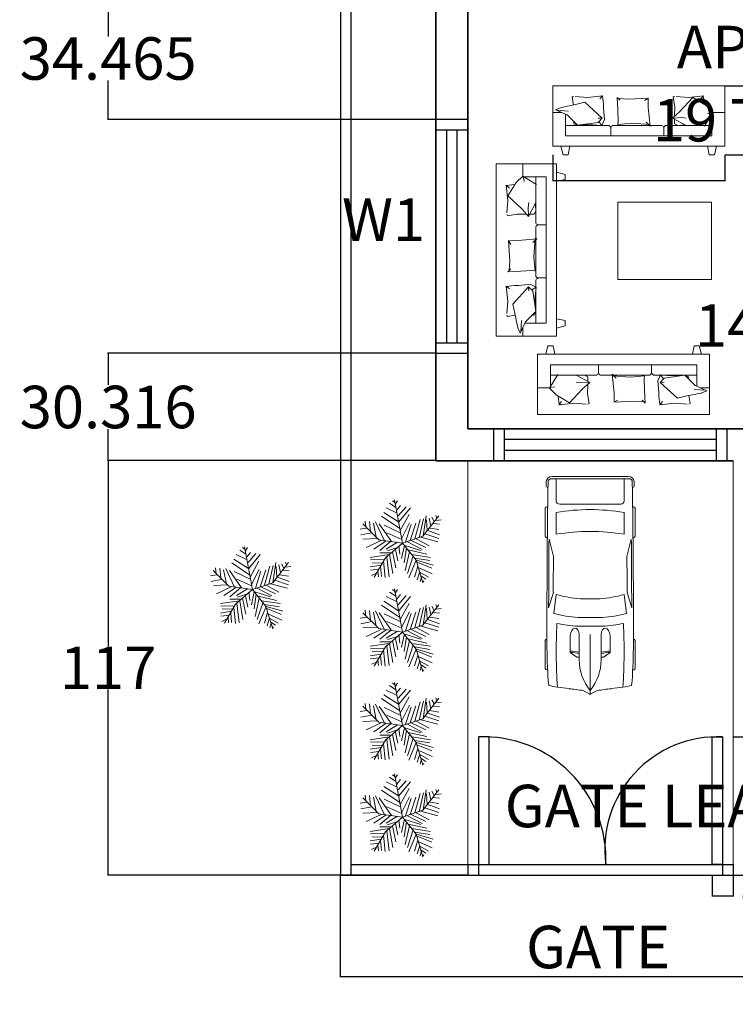
# Model space of a CAD drawing. Units: inches. Extents: x 774 to 1314, y 374 to 930.
# Tile 1 of 5: x 774 to 976, y 374 to 652. Entities that reach past the tile are written whole.
import ezdxf
from ezdxf.enums import TextEntityAlignment as Align

# ---------------------------------------------------------------- set-up
doc = ezdxf.new("R2010")
doc.units = ezdxf.units.IN
doc.header["$MEASUREMENT"] = 0
for name, color, linetype, lineweight in [('A-ANNO-DIMS', 2, 'Continuous', 18), ('A-ANNO-TEXT', 2, 'Continuous', 18), ('A-AREA-IDEN', 2, 'Continuous', 18), ('A-FURN', 8, 'Continuous', 18), ('A-GLAZ', 4, 'Continuous', 18), ('A-WALL', 1, 'Continuous', 35), ('C-PROP', 3, 'Continuous', 25), ('C-VEHC', 8, 'Continuous', 13), ('L-GATE', 6, 'Continuous', 25), ('L-PAVE', 32, 'Continuous', 18), ('L-PLNT', 3, 'Continuous', 13)]:
    doc.layers.add(name, color=color, linetype=linetype, lineweight=lineweight)
doc.layers.add('Layer4', color=4, linetype='Continuous')
doc.styles.get("Standard").update_dxf_attribs({"font": 'arial.ttf'})
doc.dimstyles.get("Standard").update_dxf_attribs({"dimtxt": 12, "dimasz": 0.18, "dimexe": 0.18, "dimexo": 0.0625, "dimgap": 0.09, "dimtad": 0, "dimtih": 1, "dimtoh": 1, "dimdec": 0, "dimzin": 0, "dimdsep": 46, "dimlunit": 4, "dimtxsty": 'Standard', "dimcen": 0.09, "dimadec": 0, "dimazin": 0, "dimtfac": 1, "dimtdec": 0, "dimtofl": 0, "dimtmove": 0, "dimatfit": 3, "dimfxl": 1, "dimtolj": 1, "dimtzin": 0, "dimarcsym": 0})

# ---------------------------------------------------------------- blocks, each defined once
blk = doc.blocks.new('tr')
at = {"layer": 'Layer4'}
for p, q in [((9, 66), (0, 66)), ((9, 63), (0, 63)), ((0, 63), (0, 3)), ((3, 63), (3, 3)), ((6, 3), (6, 63)), ((9, 3), (9, 63)), ((0, 3), (9, 3)), ((0, 0), (9, 0))]:
    blk.add_line(p, q, dxfattribs=at)
blk = doc.blocks.new('A$C684A1F33')
for p, q in [((0, 708), (1769, 708)), ((0, 708), (0, 88)), ((1769, 708), (1769, 88)), ((233, 516), (87, 486)), ((201, 592), (214, 600)), ((215, 513), (201, 592)), ((232, 599), (359, 589)), ((330, 538), (233, 516)), ((508, 377), (330, 538)), ((359, 589), (513, 606)), ((513, 606), (485, 573)), ((490, 603), (511, 604)), ((511, 604), (521, 520)), ((521, 520), (521, 475)), ((669, 458), (662, 589)), ((662, 589), (693, 560)), ((681, 577), (771, 570)), ((771, 570), (984, 581)), ((984, 581), (942, 558)), ((980, 570), (982, 484)), ((1238, 592), (1251, 600)), ((1255, 494), (1238, 592)), ((1269, 599), (1395, 589)), ((1306, 443), (1441, 588)), ((1395, 589), (1550, 606)), ((1441, 588), (1579, 505)), ((1550, 606), (1522, 573)), ((1527, 603), (1548, 604)), ((1548, 604), (1558, 520)), ((1558, 520), (1558, 518)), ((0, 434), (93, 434)), ((87, 486), (30, 462)), ((30, 462), (148, 408)), ((42, 457), (160, 448)), ((133, 415), (133, 195)), ((148, 408), (255, 302)), ((521, 475), (533, 361)), ((674, 340), (669, 458)), ((982, 484), (1001, 292)), ((1230, 377), (1306, 443)), ((1253, 397), (1255, 494)), ((1645, 436), (1559, 294)), ((1579, 505), (1645, 436)), ((1635, 429), (1590, 422)), ((1637, 434), (1637, 195)), ((1637, 434), (1769, 434)), ((216, 318), (216, 340)), ((249, 301), (216, 318)), ((313, 306), (249, 301)), ((255, 302), (467, 332)), ((409, 308), (313, 306)), ((504, 299), (409, 308)), ((498, 377), (467, 375)), ((467, 332), (508, 377)), ((504, 299), (475, 341)), ((533, 361), (504, 299)), ((669, 309), (814, 323)), ((671, 306), (674, 340)), ((814, 323), (1003, 309)), ((1001, 292), (961, 333)), ((1372, 301), (1230, 377)), ((1237, 377), (1323, 381)), ((1252, 318), (1253, 365)), ((1286, 301), (1252, 318)), ((1350, 306), (1286, 301)), ((1323, 381), (1372, 374)), ((1363, 306), (1350, 306)), ((133, 301), (576, 301)), ((598, 277), (598, 195)), ((613, 301), (1122, 301)), ((1144, 277), (1144, 195)), ((1160, 301), (1637, 301)), ((133, 195), (1637, 195)), ((0, 88), (1769, 88)), ((84, 88), (107, 0)), ((177, 88), (160, 0)), ((1592, 88), (1610, 0)), ((1685, 88), (1662, 0)), ((107, 0), (160, 0)), ((1610, 0), (1662, 0))]:
    blk.add_line(p, q)
for points, knots in [([(576, 301), (580, 299), (590, 293), (595, 283), (598, 277)], [15.247039, 15.247039, 15.247039, 15.247039, 32.166322, 53.547435, 53.547435, 53.547435, 53.547435]), ([(598, 276), (599, 282), (602, 291), (610, 298), (613, 301)], [5.353258, 5.353258, 5.353258, 5.353258, 23.098733, 39.167876, 39.167876, 39.167876, 39.167876]), ([(1122, 301), (1127, 299), (1136, 293), (1141, 283), (1144, 277)], [15.247039, 15.247039, 15.247039, 15.247039, 32.166322, 53.547435, 53.547435, 53.547435, 53.547435]), ([(1144, 276), (1145, 282), (1149, 291), (1156, 298), (1160, 301)], [5.353258, 5.353258, 5.353258, 5.353258, 23.098733, 39.167876, 39.167876, 39.167876, 39.167876])]:
    blk.add_open_spline(points, degree=3, knots=knots)
blk = doc.blocks.new('*U12')
for p, q in [((21.1, 37.41), (21.1, 36.83)), ((46.55, 38.89), (22.35, 38.89)), ((47.8, 37.39), (47.8, 37.41)), ((87.99, 31.87), (74.76, 35.92)), ((134.31, 35.6), (119.29, 31.78)), ((135.45, 37.07), (135.45, 37.41)), ((136.7, 38.89), (160.9, 38.89)), ((162.15, 37.41), (162.15, 36.77)), ((70.03, 31.54), (86.41, 29.35)), ((138.42, 29.35), (157.25, 29.35)), ((164.52, 26.39), (164.52, -26.39)), ((186.47, 29.35), (167.01, 29.35)), ((186.47, -33.5), (186.47, 33.5)), ((188.4, -32.76), (188.4, 32.76)), ((32.27, 11.63), (36.13, 17.17)), ((36.13, 17.17), (50.94, 17.17)), ((29.77, 9.51), (51.68, 9.51)), ((32.12, 9.51), (32.12, 11.15)), ((58.92, -10.77), (58.92, 10.77)), ((66.55, -10.53), (66.55, 10.53)), ((186.47, -10.53), (186.47, 10.53)), ((3.27, 6.13), (0.1, 0.41)), ((82.74, 8.5), (82.74, -8.5)), ((0, 0), (51.68, 0)), ((0.1, -0.41), (3.27, -6.13)), ((29.77, -9.51), (51.68, -9.51)), ((32.12, -9.51), (32.12, -11.15)), ((32.27, -11.63), (36.13, -17.17)), ((36.13, -17.17), (50.94, -17.17)), ((86.41, -29.35), (70.03, -31.54)), ((87.99, -31.87), (74.76, -35.92)), ((134.31, -35.6), (119.29, -31.78)), ((157.25, -29.35), (138.42, -29.35)), ((167.01, -29.35), (186.47, -29.35)), ((21.1, -37.41), (21.1, -36.83)), ((46.55, -38.89), (22.35, -38.89)), ((47.8, -37.39), (47.8, -37.41)), ((135.45, -37.07), (135.45, -37.41)), ((136.7, -38.89), (160.9, -38.89)), ((162.15, -37.41), (162.15, -36.77))]:
    blk.add_line(p, q)
for centre, major_axis, ratio, start_param, end_param in [((266.03, -27.52), (0, 313.31), 0.842304, 1.367076, 1.39176), ((41.19, -490.86), (0, 528.23), 0.842304, 0.00281, 0.075598), ((22.35, 37.41), (0, -1.48), 0.842304, 3.141593, 4.712389), ((64.48, -10555.62), (0, 10593.03), 0.842304, -0.013397, 0.002797), ((46.55, 37.41), (0, 1.48), 0.842304, -1.570796, 0), ((64.48, -10555.62), (0, -10591.55), 0.842304, 3.133765, 3.140441), ((136.7, 37.41), (0, -1.48), 0.842304, 3.141593, 4.712389), ((160.9, 37.41), (0, 1.48), 0.842304, -1.570796, 0), ((180.63, 35.84), (0, 2.22), 0.842304, -0.013017, 1.249894), ((64.48, -10556.36), (0, 10595.31), 0.842304, -0.013397, -0.013017), ((183.98, 33.5), (0, -2.96), 0.842304, 1.570796, 3.128196), ((183.98, 32.76), (0, -5.25), 0.842304, 1.570796, 3.128196), ((259.18, -27.52), (0, -305.3), 0.842304, 4.528606, 4.561838), ((37.47, -593.96), (0, -623.33), 0.842304, 3.096046, 3.200911), ((134.4, 5.39), (0, -89.78), 0.842304, 4.449482, 4.652344), ((135.29, 5.39), (0, 81.77), 0.842304, 1.245306, 1.50788), ((149.6, 2.8), (0, -79.58), 0.842304, 4.372215, 4.640744), ((95.79, -3666.35), (0, -3698.24), 0.842304, 3.134049, 3.144098), ((17.08, 0), (0, 147.02), 0.842304, 4.511394, 4.913384), ((35.91, 0), (0, 147.02), 0.842304, 4.511394, 4.913384), ((167.01, 26.39), (0, 2.96), 0.842304, 0, 1.570796), ((-204.49, 52.4), (0, -250.96), 0.842304, 1.385369, 1.434372), ((13.04, 17.01), (0, 27.42), 0.842304, 4.435146, 4.718221), ((14.2, 17.01), (0, 27.42), 0.842304, 4.435146, 4.718221), ((50.79, 13.34), (6.34, -0.36), 0.603834, -1.395552, 1.581315), ((29.77, -46.66), (0, 56.17), 0.842304, 0, 0.590319), ((32.75, 11.15), (0, 0.74), 0.842304, 0.879714, 1.570796), ((0.62, 0), (0, -0.74), 0.842304, 4.131459, 5.293319), ((-204.49, -52.4), (0, 250.96), 0.842304, -1.434372, -1.385369), ((29.77, 46.66), (0, 56.17), 0.842304, 2.551274, 3.141593), ((149.6, -2.8), (0, -79.58), 0.842304, -1.499151, -1.230623), ((32.75, -11.15), (0, -0.74), 0.842304, 4.712389, 5.403472), ((13.04, -17.01), (0, -27.42), 0.842304, 1.564964, 1.848039), ((14.2, -17.01), (0, -27.42), 0.842304, 1.564964, 1.848039), ((134.4, -5.39), (0, -89.78), 0.842304, -1.510751, -1.307889), ((135.29, -5.39), (0, -81.77), 0.842304, -1.50788, -1.245306), ((259.18, 27.52), (0, 305.3), 0.842304, 1.721348, 1.754579), ((266.03, 27.52), (0, 313.31), 0.842304, 1.749832, 1.774517), ((37.47, 593.96), (0, -623.33), 0.842304, -0.059319, 0.045547), ((95.79, 3666.35), (0, -3698.24), 0.842304, -0.002505, 0.007544), ((167.01, -26.39), (0, -2.96), 0.842304, 4.712389, 6.283185), ((183.98, -33.5), (0, 2.96), 0.842304, 3.15499, 4.712389), ((183.98, -32.76), (0, -5.25), 0.842304, 0.013397, 1.570796), ((41.19, 490.86), (0, -528.23), 0.842304, -0.075598, -0.00281), ((22.35, -37.41), (0, 1.48), 0.842304, 1.570796, 3.141593), ((64.48, 10555.62), (0, 10593.03), 0.842304, 3.138796, 3.15499), ((46.55, -37.41), (0, -1.48), 0.842304, 0, 1.570796), ((64.48, 10555.62), (0, -10591.55), 0.842304, 0.001152, 0.007828), ((136.7, -37.41), (0, -1.48), 0.842304, -1.570796, 0), ((160.9, -37.41), (0, 1.48), 0.842304, 3.141593, 4.712389), ((180.63, -35.84), (0, -2.22), 0.842304, -1.249894, 0.013017), ((64.48, 10556.36), (0, 10595.31), 0.842304, 3.15461, 3.15499)]:
    blk.add_ellipse(centre, major_axis=major_axis, ratio=ratio, start_param=start_param, end_param=end_param)
at = {"extrusion": (0, 0, -1)}
blk.add_ellipse((50.79, -13.34), major_axis=(6.34, 0.36), ratio=0.603834, start_param=-1.395552, end_param=1.581315, dxfattribs=at)
blk = doc.blocks.new('*U14')
for p, q in [((-8.737, 47.138), (-17.069, 52.711)), ((-10.186, 53.64), (-13.084, 55.962)), ((0, 0), (-10.5, 57)), ((-9.099, 51.782), (-6.563, 55.962)), ((-5.114, 28.097), (-24.676, 40.636)), ((-7.288, 39.707), (-21.778, 46.673)), ((-7.65, 43.423), (-2.578, 49.46)), ((-5.839, 35.992), (4.667, 48.067)), ((-5.114, 27.632), (10.463, 46.673)), ((-48.585, 21.131), (-49.309, 29.026)), ((-43.513, 28.561), (-42.427, 15.558)), ((-38.442, 26.239), (-34.819, 7.663)), ((-35.544, 28.097), (-24.314, 3.947)), ((-3.665, 19.273), (-27.574, 35.527)), ((-2.941, 16.486), (8.652, 37.85)), ((-1.129, 6.734), (9.014, 26.704)), ((10.101, 3.483), (17.708, 26.239)), ((16.259, 5.805), (23.142, 31.348)), ((22.055, 7.198), (27.489, 32.277)), ((27, 9), (48, 36)), ((27.127, 9.056), (31.112, 35.992)), ((31.836, 30.883), (32.561, 16.486)), ((35.096, 32.741), (37.27, 22.524)), ((38.719, 34.134), (41.979, 28.561)), ((43.791, 29.954), (51.036, 30.883)), ((44.153, 36.456), (45.239, 32.741)), ((-47.498, 19.737), (-55.83, 18.344)), ((-40.615, 13.7), (-55.105, 10.913)), ((-31.5, 4.5), (-52.5, 25.5)), ((-14.533, 2.09), (-30.834, 25.31)), ((-24.314, 23.917), (-2.941, 13.7)), ((-20.691, 13.7), (-1.129, 4.876)), ((3.942, 1.625), (11.187, 24.381)), ((33.285, 16.486), (48.862, 10.913)), ((36.183, 19.737), (48.137, 17.88)), ((40.53, 25.775), (48.862, 24.846)), ((-33.37, 6.269), (-52.207, 5.34)), ((-28.299, 3.483), (-47.86, -5.805)), ((-21.416, 3.018), (-38.079, -8.128)), ((0, 0), (-31.5, 4.5)), ((-15.982, 2.09), (-30.11, -9.521)), ((0, 0), (-22.5, -19.5)), ((-6.563, 1.161), (-21.416, -8.128)), ((0, 0), (27, 9)), ((0, 0), (18, -22.5)), ((6.478, 1.625), (26.04, -8.592)), ((11.187, 3.483), (30.749, -5.805)), ((18.07, 5.805), (35.096, -3.483)), ((24.229, 7.663), (46.688, 1.625)), ((29.662, 12.307), (48.137, 6.269)), ((-15.257, -12.772), (-30.11, -12.772)), ((-6.563, -5.805), (-19.967, -9.985)), ((-13.446, -11.378), (-8.737, -32.741)), ((-9.461, -8.592), (-6.201, -23.453)), ((-4.752, -3.483), (-3.665, -14.629)), ((2.493, -3.019), (-1.491, -20.202)), ((1.769, -2.555), (24.229, -9.521)), ((5.029, -6.27), (2.131, -25.775)), ((9.014, -11.378), (3.58, -35.992)), ((7.565, -9.056), (32.198, -14.629)), ((-17.431, -15.094), (-42.789, -18.809)), ((-24.314, -21.596), (-42.427, -22.06)), ((-26.849, -26.24), (-40.253, -25.775)), ((-22.5, -19.5), (-37.5, -45)), ((-25.038, -23.918), (-22.865, -45.281)), ((-20.691, -18.345), (-17.793, -44.352)), ((-17.069, -15.094), (-12.721, -40.172)), ((14.085, -16.951), (6.478, -40.172)), ((18.07, -22.524), (8.289, -45.745)), ((12.274, -15.094), (36.907, -18.809)), ((16.259, -19.738), (36.183, -22.989)), ((18, -22.5), (27, -52.5)), ((18.433, -22.524), (40.53, -29.026)), ((19.157, -25.311), (38.719, -33.206)), ((-28.299, -29.026), (-42.789, -31.348)), ((-30.834, -34.135), (-42.427, -35.528)), ((-32.646, -36.921), (-31.921, -44.352)), ((-29.023, -30.884), (-27.936, -43.887)), ((20.244, -30.419), (15.897, -44.816)), ((22.78, -37.85), (19.519, -48.532)), ((21.331, -32.741), (39.081, -40.636)), ((22.78, -38.314), (34.372, -44.816)), ((-34.457, -39.708), (-40.978, -42.494)), ((24.591, -45.745), (23.142, -50.854)), ((24.591, -43.423), (30.749, -47.603)), ((26.764, -49.925), (28.213, -50.854))]:
    blk.add_line(p, q)
blk = doc.blocks.new('*U16')
for p, q in [((-221.9198, 1197.3052), (-433.5526, 1338.8594)), ((-258.7244, 1362.456), (-332.3336, 1421.4348)), ((0, 0), (-266.7, 1447.8)), ((-231.1146, 1315.2628), (-166.7002, 1421.4348)), ((-129.8956, 713.6638), (-626.7704, 1032.1544)), ((-185.1152, 1008.5578), (-553.1612, 1185.4942)), ((-194.31, 1102.9442), (-65.4812, 1256.284)), ((-148.3106, 914.1968), (118.5418, 1220.9018)), ((-129.8956, 701.8528), (265.7602, 1185.4942)), ((-1234.059, 536.7274), (-1252.4486, 737.2604)), ((-1105.2302, 725.4494), (-1077.6458, 395.1732)), ((-902.8176, 713.6638), (-617.5756, 100.2538)), ((-93.091, 489.5342), (-700.3796, 902.3858)), ((-74.7014, 418.7444), (219.7608, 961.39)), ((-28.6766, 171.0436), (228.9556, 678.2816)), ((412.9786, 147.447), (587.8068, 796.2392)), ((560.197, 182.8292), (698.2206, 819.8358)), ((685.8, 228.6), (1219.2, 914.4)), ((689.0258, 230.0224), (790.2448, 914.1968)), ((808.6344, 784.4282), (827.0494, 418.7444)), ((891.4384, 831.6214), (946.658, 572.1096)), ((983.4626, 867.0036), (1066.2666, 725.4494)), ((1112.2914, 760.8316), (1296.3144, 784.4282)), ((1121.4862, 925.9824), (1149.0706, 831.6214)), ((-1206.4492, 501.3198), (-1418.082, 465.9376)), ((-1031.621, 347.98), (-1399.667, 277.1902)), ((-800.1, 114.3), (-1333.5, 647.7)), ((-976.4268, 666.4706), (-884.4026, 194.6402)), ((-369.1382, 53.086), (-783.1836, 642.874)), ((-617.5756, 607.4918), (-74.7014, 347.98)), ((-525.5514, 347.98), (-28.6766, 123.8504)), ((100.1268, 41.275), (284.1498, 619.2774)), ((256.5654, 88.4682), (449.7832, 666.4706)), ((845.439, 418.7444), (1241.0948, 277.1902)), ((919.0482, 501.3198), (1222.6798, 454.152)), ((1029.462, 654.685), (1241.0948, 631.0884)), ((-847.598, 159.2326), (-1326.0578, 135.636)), ((-718.7946, 88.4682), (-1215.644, -147.447)), ((-543.9664, 76.6572), (-967.2066, -206.4512)), ((0, 0), (-800.1, 114.3)), ((-405.9428, 53.086), (-764.794, -241.8334)), ((0, 0), (-571.5, -495.3)), ((-166.7002, 29.4894), (-543.9664, -206.4512)), ((0, 0), (685.8, 228.6)), ((0, 0), (457.2, -571.5)), ((164.5412, 41.275), (661.416, -218.2368)), ((284.1498, 88.4682), (781.0246, -147.447)), ((458.978, 147.447), (891.4384, -88.4682)), ((615.4166, 194.6402), (1185.8752, 41.275)), ((753.4148, 312.5978), (1222.6798, 159.2326)), ((-387.5278, -324.4088), (-764.794, -324.4088)), ((-166.7002, -147.447), (-507.1618, -253.619)), ((-341.5284, -289.0012), (-221.9198, -831.6214)), ((-240.3094, -218.2368), (-157.5054, -595.7062)), ((-120.7008, -88.4682), (-93.091, -371.5766)), ((63.3222, -76.6826), (-37.8714, -513.1308)), ((44.9326, -64.897), (615.4166, -241.8334)), ((127.7366, -159.258), (54.1274, -654.685)), ((228.9556, -289.0012), (90.932, -914.1968)), ((192.151, -230.0224), (817.8292, -371.5766)), ((-442.7474, -383.3876), (-1086.8406, -477.7486)), ((-617.5756, -548.5384), (-1077.6458, -560.324)), ((-681.9646, -666.496), (-1022.4262, -654.685)), ((-571.5, -495.3), (-952.5, -1143)), ((-635.9652, -607.5172), (-580.771, -1150.1374)), ((-525.5514, -465.963), (-451.9422, -1126.5408)), ((-433.5526, -383.3876), (-323.1134, -1020.3688)), ((357.759, -430.5554), (164.5412, -1020.3688)), ((458.978, -572.1096), (210.5406, -1161.923)), ((311.7596, -383.3876), (937.4378, -477.7486)), ((412.9786, -501.3452), (919.0482, -583.9206)), ((457.2, -571.5), (685.8, -1333.5)), ((468.1982, -572.1096), (1029.462, -737.2604)), ((486.5878, -642.8994), (983.4626, -843.4324)), ((-718.7946, -737.2604), (-1086.8406, -796.2392)), ((-783.1836, -867.029), (-1077.6458, -902.4112)), ((-829.2084, -937.7934), (-810.7934, -1126.5408)), ((-737.1842, -784.4536), (-709.5744, -1114.7298)), ((514.1976, -772.6426), (403.7838, -1138.3264)), ((578.612, -961.39), (495.7826, -1232.7128)), ((541.8074, -831.6214), (992.6574, -1032.1544)), ((578.612, -973.1756), (873.0488, -1138.3264)), ((-875.2078, -1008.5832), (-1040.8412, -1079.3476)), ((624.6114, -1161.923), (587.8068, -1291.6916)), ((624.6114, -1102.9442), (781.0246, -1209.1162)), ((679.8056, -1268.095), (716.6102, -1291.6916))]:
    blk.add_line(p, q)
blk = doc.blocks.new('GATE-LEAF-36IN')
for p, q in [((3, 3), (3, 0)), ((6, 3), (6, 0))]:
    blk.add_line(p, q)
blk.add_lwpolyline([(3, 3), (0, 3), (0, 39), (3, 39)], close=True)
blk = doc.blocks.new('*D33')
at = {"layer": 'A-ANNO-DIMS', "color": 0, "lineweight": -2, "transparency": 16777216}
for p, q in [((975.4, 449.57), (981.36, 449.57)), ((981.18, 449.39), (981.18, 436.36)), ((981.18, 410.75), (981.18, 423.77)), ((975.4, 410.57), (981.36, 410.57))]:
    blk.add_line(p, q, dxfattribs=at)
at = {"layer": 'A-ANNO-DIMS', "color": 0, "transparency": 16777216}
for points in [[(981.15, 449.39), (981.21, 449.39), (981.18, 449.57)], [(981.15, 410.75), (981.21, 410.75), (981.18, 410.57)]]:
    blk.add_solid(points, dxfattribs=at)
at = {"layer": 'Defpoints', "color": 0, "transparency": 16777216}
for p in [(975.33, 449.57), (981.18, 449.57), (975.33, 410.57)]:
    blk.add_point(p, dxfattribs=at)
at = {"layer": 'A-ANNO-DIMS', "color": 0, "transparency": 16777216, "insert": (981.18, 430.07), "char_height": 12, "attachment_point": 5}
blk.add_mtext('\\A1;GATE LEAF 39 TYP.', dxfattribs=at)
blk = doc.blocks.new('*D34')
at = {"layer": 'A-ANNO-DIMS', "color": 0, "lineweight": -2, "transparency": 16777216}
for p, q in [((969.33, 410.5), (969.33, 404.54)), ((975.33, 410.5), (975.33, 404.54)), ((969.51, 404.72), (975.15, 404.72)), ((975.33, 404.72), (975.51, 404.72))]:
    blk.add_line(p, q, dxfattribs=at)
at = {"layer": 'A-ANNO-DIMS', "color": 0, "transparency": 16777216}
for points in [[(969.51, 404.75), (969.51, 404.69), (969.33, 404.72)], [(975.15, 404.75), (975.15, 404.69), (975.33, 404.72)]]:
    blk.add_solid(points, dxfattribs=at)
at = {"layer": 'Defpoints', "color": 0, "transparency": 16777216}
for p in [(969.33, 410.57), (975.33, 410.57), (975.33, 404.72)]:
    blk.add_point(p, dxfattribs=at)
at = {"layer": 'A-ANNO-DIMS', "color": 0, "transparency": 16777216, "insert": (1000.18, 404.72), "char_height": 12, "attachment_point": 5}
blk.add_mtext('\\A1;6 TYP.', dxfattribs=at)
blk = doc.blocks.new('*D37')
at = {"layer": 'A-ANNO-DIMS', "color": 0, "lineweight": -2, "transparency": 16777216}
for p, q in [((924.33, 613.89), (924.33, 606.48)), ((972.96, 613.89), (972.96, 606.48)), ((924.51, 606.66), (972.78, 606.66)), ((972.96, 606.66), (973.14, 606.66))]:
    blk.add_line(p, q, dxfattribs=at)
at = {"layer": 'A-ANNO-DIMS', "color": 0, "transparency": 16777216}
for points in [[(924.51, 606.69), (924.51, 606.63), (924.33, 606.66)], [(972.78, 606.69), (972.78, 606.63), (972.96, 606.66)]]:
    blk.add_solid(points, dxfattribs=at)
at = {"layer": 'Defpoints', "color": 0, "transparency": 16777216}
for p in [(924.33, 613.95), (972.96, 613.95), (972.96, 606.66)]:
    blk.add_point(p, dxfattribs=at)
at = {"layer": 'A-ANNO-DIMS', "color": 0, "transparency": 16777216, "insert": (1027.55, 606.66), "char_height": 12, "attachment_point": 5}
blk.add_mtext('\\A1;SOFA 49 TYP.', dxfattribs=at)
blk = doc.blocks.new('*D38')
at = {"layer": 'A-ANNO-DIMS', "color": 0, "lineweight": -2, "transparency": 16777216}
for p, q in [((973.02, 633.4), (980.43, 633.4)), ((980.25, 633.22), (980.25, 629.89)), ((980.25, 614.13), (980.25, 617.46)), ((973.02, 613.95), (980.43, 613.95))]:
    blk.add_line(p, q, dxfattribs=at)
at = {"layer": 'A-ANNO-DIMS', "color": 0, "transparency": 16777216}
for points in [[(980.22, 633.22), (980.28, 633.22), (980.25, 633.4)], [(980.22, 614.13), (980.28, 614.13), (980.25, 613.95)]]:
    blk.add_solid(points, dxfattribs=at)
at = {"layer": 'Defpoints', "color": 0, "transparency": 16777216}
for p in [(972.96, 633.4), (980.25, 633.4), (972.96, 613.95)]:
    blk.add_point(p, dxfattribs=at)
at = {"layer": 'A-ANNO-DIMS', "color": 0, "transparency": 16777216, "insert": (980.25, 623.68), "char_height": 12, "attachment_point": 5}
blk.add_mtext('\\A1;19 TYP.', dxfattribs=at)
blk = doc.blocks.new('*D51')
at = {"layer": 'A-ANNO-DIMS', "color": 0, "lineweight": -2, "transparency": 16777216}
for p, q in [((1072.03, 644.35), (1071.85, 644.35)), ((1072.03, 640.32), (1072.03, 644.53)), ((1099.12, 644.35), (1072.21, 644.35)), ((1099.3, 640.32), (1099.3, 644.53))]:
    blk.add_line(p, q, dxfattribs=at)
at = {"layer": 'A-ANNO-DIMS', "color": 0, "transparency": 16777216}
for points in [[(1072.21, 644.38), (1072.21, 644.32), (1072.03, 644.35)], [(1099.12, 644.38), (1099.12, 644.32), (1099.3, 644.35)]]:
    blk.add_solid(points, dxfattribs=at)
at = {"layer": 'Defpoints', "color": 0, "transparency": 16777216}
for p in [(1072.03, 644.35), (1072.03, 640.25), (1099.3, 640.25)]:
    blk.add_point(p, dxfattribs=at)
at = {"layer": 'A-ANNO-DIMS', "color": 0, "transparency": 16777216, "insert": (1013.43, 644.35), "char_height": 12, "attachment_point": 5}
blk.add_mtext('\\A1;APPLIANCE 27', dxfattribs=at)
blk = doc.blocks.new('*D53')
at = {"layer": 'A-ANNO-DIMS', "color": 0, "lineweight": -2, "transparency": 16777216}
for p, q in [((864.33, 410.5), (864.33, 381.78)), ((1230.33, 410.5), (1230.33, 381.78)), ((864.51, 381.96), (1034, 381.96)), ((1230.15, 381.96), (1060.67, 381.96))]:
    blk.add_line(p, q, dxfattribs=at)
at = {"layer": 'A-ANNO-DIMS', "color": 0, "transparency": 16777216}
for points in [[(864.51, 381.99), (864.51, 381.93), (864.33, 381.96)], [(1230.15, 381.99), (1230.15, 381.93), (1230.33, 381.96)]]:
    blk.add_solid(points, dxfattribs=at)
at = {"layer": 'Defpoints', "color": 0, "transparency": 16777216}
for p in [(864.33, 410.57), (1230.33, 410.57), (1230.33, 381.96)]:
    blk.add_point(p, dxfattribs=at)
at = {"layer": 'A-ANNO-DIMS', "color": 0, "transparency": 16777216, "insert": (1047.33, 381.96), "char_height": 12, "attachment_point": 5}
blk.add_mtext('\\A1;366', dxfattribs=at)
blk = doc.blocks.new('*D61')
at = {"layer": 'A-ANNO-DIMS', "color": 0, "lineweight": -2, "transparency": 16777216}
for p, q in [((891.27, 527.57), (798.56, 527.57)), ((798.74, 527.39), (798.74, 475.18)), ((798.74, 410.75), (798.74, 462.95)), ((900.27, 410.57), (798.56, 410.57))]:
    blk.add_line(p, q, dxfattribs=at)
at = {"layer": 'A-ANNO-DIMS', "color": 0, "transparency": 16777216}
for points in [[(798.71, 527.39), (798.77, 527.39), (798.74, 527.57)], [(798.71, 410.75), (798.77, 410.75), (798.74, 410.57)]]:
    blk.add_solid(points, dxfattribs=at)
at = {"layer": 'Defpoints', "color": 0, "transparency": 16777216}
for p in [(798.74, 527.57), (891.33, 527.57), (900.33, 410.57)]:
    blk.add_point(p, dxfattribs=at)
at = {"layer": 'A-ANNO-DIMS', "color": 0, "transparency": 16777216, "insert": (798.74, 469.07), "char_height": 12, "attachment_point": 5}
blk.add_mtext('\\A1;117', dxfattribs=at)
blk = doc.blocks.new('*D62')
at = {"layer": 'A-ANNO-DIMS', "color": 0, "lineweight": -2, "transparency": 16777216}
for p, q in [((891.27, 557.88), (798.56, 557.88)), ((798.74, 557.7), (798.74, 548.94)), ((798.74, 527.75), (798.74, 536.5)), ((891.27, 527.57), (798.56, 527.57))]:
    blk.add_line(p, q, dxfattribs=at)
at = {"layer": 'A-ANNO-DIMS', "color": 0, "transparency": 16777216}
for points in [[(798.71, 557.7), (798.77, 557.7), (798.74, 557.88)], [(798.71, 527.75), (798.77, 527.75), (798.74, 527.57)]]:
    blk.add_solid(points, dxfattribs=at)
at = {"layer": 'Defpoints', "color": 0, "transparency": 16777216}
for p in [(798.74, 557.88), (891.33, 557.88), (891.33, 527.57)]:
    blk.add_point(p, dxfattribs=at)
at = {"layer": 'A-ANNO-DIMS', "color": 0, "transparency": 16777216, "insert": (798.74, 542.72), "char_height": 12, "attachment_point": 5}
blk.add_mtext('\\A1;30.316', dxfattribs=at)
blk = doc.blocks.new('*D63')
at = {"layer": 'A-ANNO-DIMS', "color": 0, "lineweight": -2, "transparency": 16777216}
for p, q in [((891.27, 658.35), (798.56, 658.35)), ((798.74, 658.17), (798.74, 647.34)), ((798.74, 624.06), (798.74, 634.89)), ((891.27, 623.88), (798.56, 623.88))]:
    blk.add_line(p, q, dxfattribs=at)
at = {"layer": 'A-ANNO-DIMS', "color": 0, "transparency": 16777216}
for points in [[(798.71, 658.17), (798.77, 658.17), (798.74, 658.35)], [(798.71, 624.06), (798.77, 624.06), (798.74, 623.88)]]:
    blk.add_solid(points, dxfattribs=at)
at = {"layer": 'Defpoints', "color": 0, "transparency": 16777216}
for p in [(798.74, 658.35), (891.33, 658.35), (891.33, 623.88)]:
    blk.add_point(p, dxfattribs=at)
at = {"layer": 'A-ANNO-DIMS', "color": 0, "transparency": 16777216, "insert": (798.74, 641.11), "char_height": 12, "attachment_point": 5}
blk.add_mtext('\\A1;34.465', dxfattribs=at)

msp = doc.modelspace()

# ---------------------------------------------------------------- linework, layer by layer
at = {"layer": 'A-FURN'}
msp.add_lwpolyline([(942.7268, 578.7015), (969.1941, 578.7015), (969.1941, 600.5862), (942.7268, 600.5862)], close=True, dxfattribs=at)
at = {"layer": 'A-WALL'}
for p, q in [((900.3347, 734.5656), (900.3347, 536.5656)), ((984.3347, 536.5656), (900.3347, 536.5656)), ((975.3347, 527.5656), (891.3347, 527.5656))]:
    msp.add_line(p, q, dxfattribs=at)
msp.add_lwpolyline([(1203.3347, 740.5656), (1203.3347, 869.5656), (891.3347, 869.5656), (891.3347, 527.5656)], dxfattribs=at)
at = {"layer": 'C-PROP'}
msp.add_line((867.3347, 413.5656), (867.3347, 410.5656), dxfattribs=at)
msp.add_lwpolyline([(864.3347, 410.5656), (1230.3347, 410.5656), (1230.3347, 896.5656), (864.3347, 896.5656)], close=True, dxfattribs=at)
for points in [[(1227.3347, 740.5656), (1227.3347, 893.5656), (867.3347, 893.5656), (867.3347, 413.5656), (975.3347, 413.5656)], [(900.3347, 413.5656), (975.3347, 413.5656)]]:
    msp.add_lwpolyline(points, dxfattribs=at)
at = {"layer": 'L-GATE'}
for centre, radius, start, end in [((904.8347, 415.0656), 34.5326, 357.510447, 92.489553), ((970.8347, 417.8156), 31.7854, 87.295124, 187.683982)]:
    msp.add_arc(centre, radius, start, end, dxfattribs=at)
at = {"layer": 'L-PAVE'}
for p, q in [((900.3347, 527.5656), (900.3347, 413.5656)), ((975.3347, 413.5656), (975.3347, 527.5656))]:
    msp.add_line(p, q, dxfattribs=at)

# ---------------------------------------------------------------- block references
at = {"layer": 'A-FURN', "xscale": 0.0274825048750847, "yscale": 0.0274825048750847, "zscale": 0.0274825048750847}
msp.add_blockref('A$C684A1F33', (924.3264, 613.9496), dxfattribs=at)
for p, rotation in [((927.8424, 562.7095), 90), ((968.6583, 560.0203), 180.0000000000001)]:
    msp.add_blockref('A$C684A1F33', p, dxfattribs=dict(at, rotation=rotation))
at = {"layer": 'A-GLAZ'}
msp.add_blockref('tr', (891.3347, 557.8818), dxfattribs=at)
at = {"layer": 'A-GLAZ', "rotation": 270}
msp.add_blockref('tr', (907.6221, 536.5656), dxfattribs=at)
at = {"layer": 'C-VEHC', "xscale": 0.3265334135073655, "yscale": 0.3265334135073655, "zscale": 0.3265334135073655, "rotation": 90}
msp.add_blockref('*U12', (934.9117, 461.5901), dxfattribs=at)
at = {"layer": 'L-GATE', "extrusion": (0, 0, -1), "zscale": -1}
msp.add_blockref('GATE-LEAF-36IN', (-906.3344, 410.566), dxfattribs=at)
at = {"layer": 'L-GATE'}
msp.add_blockref('GATE-LEAF-36IN', (969.335, 410.566), dxfattribs=at)
at = {"layer": 'L-PLNT'}
for name, p, xscale, yscale, zscale in [('*U14', (881.9018, 504.2867), 0.213927632294721, 0.213927632294721, 0.213927632294721), ('*U16', (839.5093, 491.185), 0.00833239555031, 0.00833239555031, 0.00833239555031), ('*U14', (881.9018, 479.1937), 0.213927632294721, 0.213927632294721, 0.213927632294721), ('*U14', (881.9018, 452.7875), 0.213927632294721, 0.213927632294721, 0.213927632294721), ('*U14', (881.9018, 426.9307), 0.213927632294721, 0.213927632294721, 0.213927632294721)]:
    msp.add_blockref(name, p, dxfattribs=dict(at, xscale=xscale, yscale=yscale, zscale=zscale))

# ---------------------------------------------------------------- texts
at = {"layer": 'A-ANNO-TEXT'}
for s, p in [('W1', (876.5499, 589.5941)), ('GATE', (937.1415, 384.265))]:
    msp.add_text(s, height=12, dxfattribs=at).set_placement(p, align=Align.CENTER)
at = {"layer": 'A-AREA-IDEN'}
msp.add_text('14\'6"X12\'', height=12, dxfattribs=at).set_placement((1000.3471, 559.7474), align=Align.CENTER)

# ---------------------------------------------------------------- dimensions: what is measured, and where the dimension line sits
at = {"layer": 'A-ANNO-DIMS'}
for base, p1, p2, angle, text, picture, middle in [((1072.0264, 644.3458), (1099.3039, 640.2542), (1072.0264, 640.2542), 180, 'APPLIANCE <>', '*D51', (1013.4345, 644.3458)), ((980.2504, 633.4014), (972.9559, 613.9496), (972.9559, 633.4014), 90, '<> TYP.', '*D38', (980.2504, 623.6755)), ((981.1847, 449.5656), (975.3347, 410.5656), (975.3347, 449.5656), 90, 'GATE LEAF <> TYP.', '*D33', (981.1847, 430.0656))]:
    dim = msp.add_linear_dim(base=base, p1=p1, p2=p2, angle=angle, text=text, dimstyle='Standard', override={"dimdec": 0, "dimlfac": 1, "dimrnd": 0, "dimzin": 0, "dimdsep": 46, "dimlunit": 2}, dxfattribs=at)
    dim.commit()
    dim.dimension.update_dxf_attribs({"geometry": picture, "text_midpoint": middle})
for base, p1, p2, override, picture, middle in [((798.7384, 658.3472), (891.3347, 623.8818), (891.3347, 658.3472), {"dimdec": 3, "dimlfac": 1, "dimrnd": 0, "dimzin": 0, "dimdsep": 46, "dimlunit": 2}, '*D63', (798.7384, 641.1145)), ((798.7384, 557.8818), (891.3347, 527.5656), (891.3347, 557.8818), {"dimdec": 3, "dimlfac": 1, "dimrnd": 0, "dimzin": 0, "dimdsep": 46, "dimlunit": 2}, '*D62', (798.7384, 542.7237)), ((798.7384, 527.5656), (900.3347, 410.5656), (891.3347, 527.5656), {"dimdec": 0, "dimlfac": 1, "dimrnd": 0, "dimzin": 0, "dimdsep": 46, "dimlunit": 2}, '*D61', (798.7384, 469.0656))]:
    dim = msp.add_linear_dim(base=base, p1=p1, p2=p2, angle=90, dimstyle='Standard', override=override, dxfattribs=at)
    dim.commit()
    dim.dimension.update_dxf_attribs({"geometry": picture, "text_midpoint": middle})
for base, p1, p2, text, picture, middle in [((972.9559, 606.6552), (924.3264, 613.9496), (972.9559, 613.9496), 'SOFA <> TYP.', '*D37', (1027.5533, 606.6552)), ((975.3347, 404.7156), (969.3347, 410.5656), (975.3347, 410.5656), '<> TYP.', '*D34', (1000.1818, 404.7156))]:
    dim = msp.add_linear_dim(base=base, p1=p1, p2=p2, text=text, dimstyle='Standard', override={"dimdec": 0, "dimlfac": 1, "dimrnd": 0, "dimzin": 0, "dimdsep": 46, "dimlunit": 2}, dxfattribs=at)
    dim.commit()
    dim.dimension.update_dxf_attribs({"geometry": picture, "text_midpoint": middle})
dim = msp.add_linear_dim(base=(1230.3347, 381.9636), p1=(864.3347, 410.5656), p2=(1230.3347, 410.5656), dimstyle='Standard', override={"dimdec": 0, "dimlfac": 1, "dimrnd": 0, "dimzin": 0, "dimdsep": 46, "dimlunit": 2}, dxfattribs=at)
dim.commit()
dim.dimension.update_dxf_attribs({"geometry": '*D53', "text_midpoint": (1047.3347, 381.9636)})

doc.saveas('drawing.dxf')
